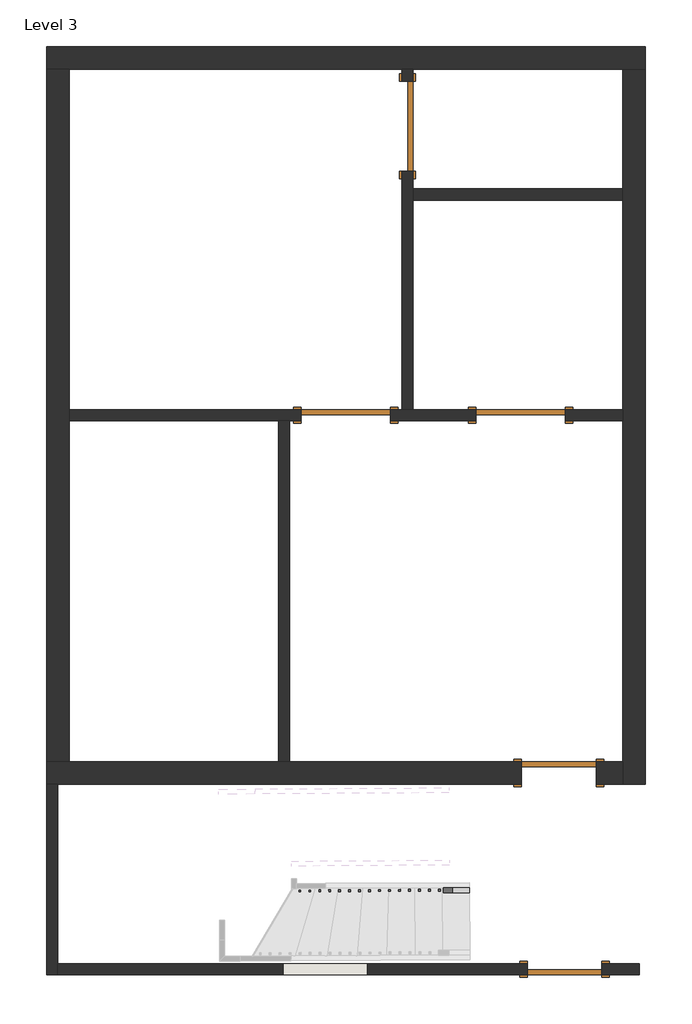
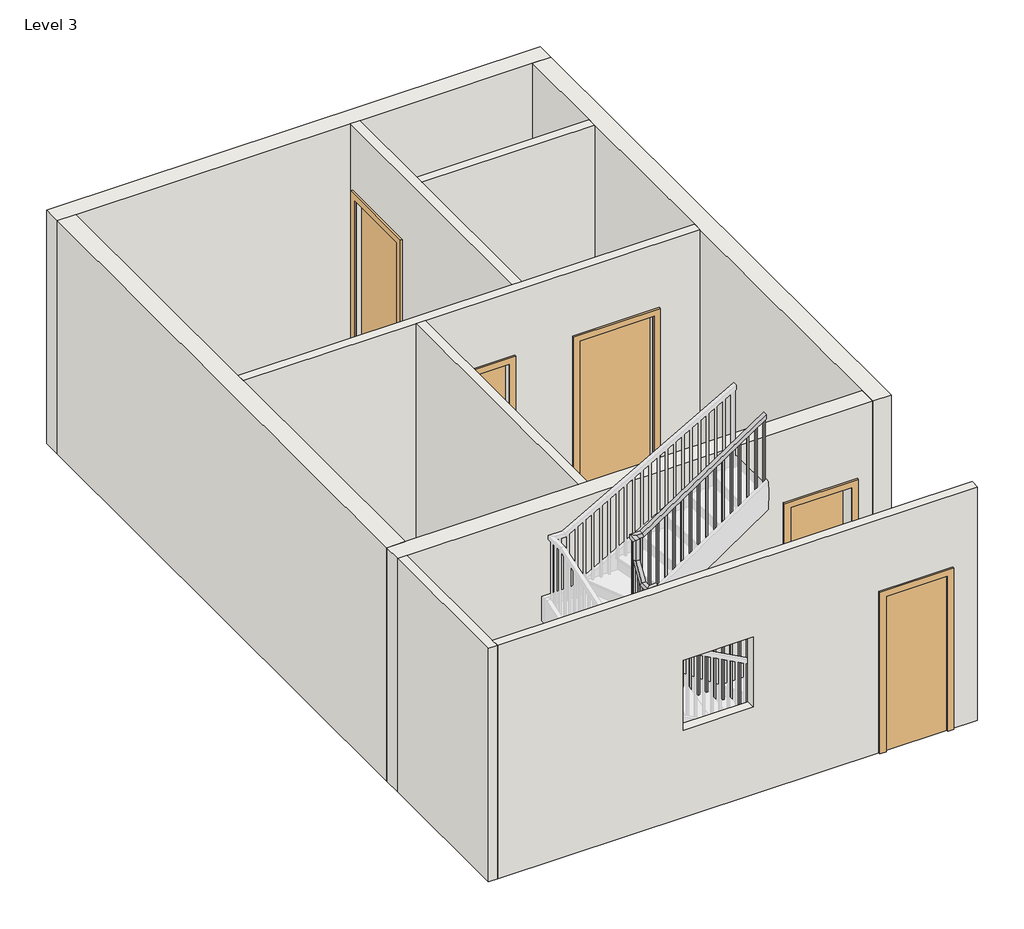
# One storey, part 1 of 2: 10 walls, 5 doors, 1 railing.
"""IFC4 building model written with IfcOpenShell, lengths in millimetres."""

from ifc_helpers import new_model, si_unit, frame, origin, place, context, project, spatial, polyline, outline, extrude, faceted_brep, transform, mapped, element, save
from components import door_a1484949, door_d8f5dbb5, door_e5f9f3c4, door_305aa2a5

model = new_model("IFC4")

# Units and contexts
model_context = context("Model", 3, world=origin())
ifc_project = project(units=[si_unit("LENGTHUNIT", "METRE", prefix="MILLI")], contexts=[model_context])

# Site, building, storey
site = spatial("IfcSite", under=ifc_project)
building = spatial("IfcBuilding", under=site)
storey = spatial("IfcBuildingStorey", under=building, Name="Level 3", Elevation=3200.4)

# Doors
placement = place(None, origin())
door_shape = door_a1484949(model_context)
element("IfcDoor", 1, ObjectType="Single-Flush : 30\" x 80\"", at=placement, inside=storey, context=model_context, shape_type="MappedRepresentation", body=[
    mapped(door_shape, transform((792.5410386, -2372.0109248, 3200.4), x_axis=(1.0, 0.0, 0.0), y_axis=(0.0, 1.0, 0.0), z_axis=(0.0, 0.0, 1.0))),
])
door_2_shape = door_d8f5dbb5(model_context)
element("IfcDoor", 2, ObjectType="Single-Flush : 30\" x 80\"", at=placement, inside=storey, context=model_context, shape_type="MappedRepresentation", body=[
    mapped(door_2_shape, transform((849.6910386, -4372.2609248, 3200.4), x_axis=(-1.0, 0.0, 0.0), y_axis=(0.0, -1.0, 0.0), z_axis=(0.0, 0.0, 1.0))),
])
door_3_shape = door_e5f9f3c4(model_context)
element("IfcDoor", 3, ObjectType="Single-Flush : 36\" x 84\"", at=placement, inside=storey, context=model_context, shape_type="MappedRepresentation", body=[
    mapped(door_3_shape, transform((-750.5089614, 4209.7640752, 3200.4), x_axis=(0.0, -1.0, 0.0), y_axis=(1.0, 0.0, 0.0), z_axis=(0.0, 0.0, 1.0))),
])
door_4_shape = door_305aa2a5(model_context)
element("IfcDoor", 4, ObjectType="Single-Flush : 36\" x 84\"", at=placement, inside=storey, context=model_context, shape_type="MappedRepresentation", body=[
    mapped(door_4_shape, transform((402.0160386, 1266.5390752, 3200.4), x_axis=(-1.0, 0.0, 0.0), y_axis=(0.0, -1.0, 0.0), z_axis=(0.0, 0.0, 1.0))),
])
element("IfcDoor", 5, ObjectType="Single-Flush : 36\" x 84\"", at=placement, inside=storey, context=model_context, shape_type="MappedRepresentation", body=[
    mapped(door_4_shape, transform((-1379.1589614, 1266.5390752, 3200.4), x_axis=(-1.0, 0.0, 0.0), y_axis=(0.0, -1.0, 0.0), z_axis=(0.0, 0.0, 1.0))),
])

# Railing
element("IfcRailing", 6, ObjectType="Handrail - Rectangular", at=placement, inside=storey, context=model_context, shape_type="SolidModel", body=[
    faceted_brep([(-120.3816305, -3590.4209536, 4284.1333333), (-120.3816305, -3590.4209536, 4222.9630107), (-120.6930289, -3539.621908, 4222.9630107), (-120.6930289, -3539.621908, 4284.1333333), (-1854.5612186, -3601.0514854, 5447.4182998), (-1905.3602642, -3601.3628839, 5420.3238978), (-1905.6716627, -3550.5638383, 5420.3238978), (-1854.8726171, -3550.2524399, 5447.4182998), (-1854.5612186, -3601.0514854, 5669.6829276), (-1905.3602642, -3601.3628839, 5618.8829276), (-1905.6716627, -3550.5638383, 5618.8829276), (-1854.8726171, -3550.2524399, 5669.6829276), (-1981.5588325, -3601.8299816, 5669.6829276), (-1981.5588325, -3601.8299816, 5618.8829276), (-1931.0711854, -3550.7195376, 5618.8829276), (-1931.0711854, -3550.7195376, 5669.6829276), (-1982.3373287, -3474.8323677, 5669.6829276), (-1982.5128182, -3446.2044317, 5618.8829276), (-1931.7137726, -3445.8930332, 5618.8829276), (-1931.5382832, -3474.5209692, 5669.6829276), (-1983.1158249, -3347.8347538, 5879.4434812), (-1983.4272234, -3297.0357082, 5865.2632575), (-1932.6281778, -3296.7243097, 5865.2632575), (-1932.3167793, -3347.5233553, 5879.4434812), (-1983.1158249, -3347.8347538, 6150.8951436), (-1983.4272234, -3297.0357082, 6100.0951436), (-1932.6281778, -3296.7243097, 6100.0951436), (-1932.3167793, -3347.5233553, 6150.8951436), (-1983.8943211, -3220.8371398, 6150.8951436), (-1983.8943211, -3220.8371398, 6100.0951436), (-1932.783877, -3271.3247869, 6100.0951436), (-1932.783877, -3271.3247869, 6150.8951436), (-1856.8967072, -3220.0586437, 6150.8951436), (-1841.6341703, -3219.9650842, 6100.0951436), (-1841.3227719, -3270.7641298, 6100.0951436), (-1856.5853087, -3270.8576892, 6150.8951436), (-324.9523945, -3210.6678153, 7162.8), (-324.6409961, -3261.4668609, 7162.8), (-324.6409961, -3261.4668609, 7101.9185401), (-324.9523945, -3210.6678153, 7101.9185401)], [[[0, 1, 2, 3]], [[1, 0, 4, 5]], [[2, 1, 5, 6]], [[3, 2, 6, 7]], [[0, 3, 7, 4]], [[5, 4, 8, 9]], [[6, 5, 9, 10]], [[7, 6, 10, 11]], [[4, 7, 11, 8]], [[9, 8, 12, 13]], [[10, 9, 13, 14]], [[11, 10, 14, 15]], [[8, 11, 15, 12]], [[13, 12, 16, 17]], [[14, 13, 17, 18]], [[15, 14, 18, 19]], [[12, 15, 19, 16]], [[17, 16, 20, 21]], [[18, 17, 21, 22]], [[19, 18, 22, 23]], [[16, 19, 23, 20]], [[21, 20, 24, 25]], [[22, 21, 25, 26]], [[23, 22, 26, 27]], [[20, 23, 27, 24]], [[25, 24, 28, 29]], [[26, 25, 29, 30]], [[27, 26, 30, 31]], [[24, 27, 31, 28]], [[29, 28, 32, 33]], [[30, 29, 33, 34]], [[31, 30, 34, 35]], [[28, 31, 35, 32]], [[36, 37, 38, 39]], [[33, 32, 36, 39]], [[34, 33, 39, 38]], [[35, 34, 38, 37]], [[32, 35, 37, 36]]]),
    extrude(outline(polyline([(222.3085098, -19.05), (234.8914903, 0.0), (1246.1854534, 0.0), (1246.1854534, -19.05), (222.3085098, -19.05)])), frame((-342.2360746, -3245.6994205, 7325.2521201), z_axis=(-0.00612989118043648, 0.9999812120405643, 0.0), x_axis=(0.0, 0.0, -1.0)), (0.0, 0.0, 1.0), 19.05),
    extrude(outline(polyline([(222.3085098, -19.0499999), (234.8914902, 0.0), (1179.0762243, 0.0), (1179.0762243, -19.0499999), (222.3085098, -19.0499999)])), frame((-443.8341657, -3246.3222175, 7258.142891), z_axis=(-0.00612989118043648, 0.9999812120405643, 0.0), x_axis=(0.0, 0.0, -1.0)), (0.0, 0.0, 1.0), 19.05),
    extrude(outline(polyline([(222.3085098, -19.05), (234.8914902, 0.0), (1111.9669952, 0.0), (1111.9669952, -19.05), (222.3085098, -19.05)])), frame((-545.4322569, -3246.9450144, 7191.0336619), z_axis=(-0.00612989118043648, 0.9999812120405643, 0.0), x_axis=(0.0, 0.0, -1.0)), (0.0, 0.0, 1.0), 19.05),
    extrude(outline(polyline([(222.3085098, -19.05), (234.8914902, 0.0), (1214.1910995, 0.0), (1214.1910995, -19.05), (222.3085098, -19.05)])), frame((-647.030348, -3247.5678114, 7123.9244328), z_axis=(-0.00612989118043648, 0.9999812120405643, 0.0), x_axis=(0.0, 0.0, -1.0)), (0.0, 0.0, 1.0), 19.05),
    extrude(outline(polyline([(222.3085098, -19.05), (234.8914902, 0.0), (1147.0818704, 0.0), (1147.0818704, -19.05), (222.3085098, -19.05)])), frame((-748.6284392, -3248.1906083, 7056.8152037), z_axis=(-0.00612989118043648, 0.9999812120405643, 0.0), x_axis=(0.0, 0.0, -1.0)), (0.0, 0.0, 1.0), 19.05),
    extrude(outline(polyline([(222.3085098, -19.05), (234.8914902, 0.0), (1079.9726413, 0.0), (1079.9726413, -19.05), (222.3085098, -19.05)])), frame((-850.2265303, -3248.8134053, 6989.7059746), z_axis=(-0.00612989118043648, 0.9999812120405643, 0.0), x_axis=(0.0, 0.0, -1.0)), (0.0, 0.0, 1.0), 19.05),
    extrude(outline(polyline([(222.3085098, -19.05), (234.8914902, 0.0), (1182.1967455, 0.0), (1182.1967455, -19.05), (222.3085098, -19.05)])), frame((-951.8246215, -3249.4362022, 6922.5967455), z_axis=(-0.00612989118043648, 0.9999812120405643, 0.0), x_axis=(0.0, 0.0, -1.0)), (0.0, 0.0, 1.0), 19.05),
    extrude(outline(polyline([(222.3085097, -19.05), (234.8914902, 0.0), (1115.0875164, 0.0), (1115.0875164, -19.05), (222.3085097, -19.05)])), frame((-1053.4227126, -3250.0589992, 6855.4875164), z_axis=(-0.00612989118043648, 0.9999812120405643, 0.0), x_axis=(0.0, 0.0, -1.0)), (0.0, 0.0, 1.0), 19.05),
    extrude(outline(polyline([(222.3085097, -19.0499999), (234.8914902, 0.0), (1047.9782873, 0.0), (1047.9782873, -19.0499999), (222.3085097, -19.0499999)])), frame((-1155.0208037, -3250.6817961, 6788.3782873), z_axis=(-0.00612989118043648, 0.9999812120405643, 0.0), x_axis=(0.0, 0.0, -1.0)), (0.0, 0.0, 1.0), 19.05),
    extrude(outline(polyline([(222.3085097, -19.05), (234.8914902, 0.0), (1150.2023915, 0.0), (1150.2023915, -19.05), (222.3085097, -19.05)])), frame((-1256.6188949, -3251.304593, 6721.2690582), z_axis=(-0.00612989118043648, 0.9999812120405643, 0.0), x_axis=(0.0, 0.0, -1.0)), (0.0, 0.0, 1.0), 19.05),
    extrude(outline(polyline([(222.3085098, -19.05), (234.8914903, 0.0), (1083.0931625, 0.0), (1083.0931625, -19.05), (222.3085098, -19.05)])), frame((-1358.216986, -3251.92739, 6654.1598292), z_axis=(-0.00612989118043648, 0.9999812120405643, 0.0), x_axis=(0.0, 0.0, -1.0)), (0.0, 0.0, 1.0), 19.05),
    extrude(outline(polyline([(222.3085098, -19.05), (234.8914903, 0.0), (1185.3172668, 0.0), (1185.3172668, -19.05), (222.3085098, -19.05)])), frame((-1459.8150772, -3252.5501869, 6587.0506001), z_axis=(-0.00612989118043648, 0.9999812120405643, 0.0), x_axis=(0.0, 0.0, -1.0)), (0.0, 0.0, 1.0), 19.05),
    extrude(outline(polyline([(222.3085098, -19.05), (234.8914903, 0.0), (1118.2080377, 0.0), (1118.2080377, -19.05), (222.3085098, -19.05)])), frame((-1561.4131683, -3253.1729839, 6519.941371), z_axis=(-0.00612989118043648, 0.9999812120405643, 0.0), x_axis=(0.0, 0.0, -1.0)), (0.0, 0.0, 1.0), 19.05),
    extrude(outline(polyline([(222.3085098, -19.05), (234.8914902, 0.0), (1051.0988086, 0.0), (1051.0988086, -19.05), (222.3085098, -19.05)])), frame((-1663.0112595, -3253.7957808, 6452.8321419), z_axis=(-0.00612989118043648, 0.9999812120405643, 0.0), x_axis=(0.0, 0.0, -1.0)), (0.0, 0.0, 1.0), 19.05),
    extrude(outline(polyline([(222.3085098, -19.05), (234.8914902, 0.0), (1153.3229128, 0.0), (1153.3229128, -19.05), (222.3085098, -19.05)])), frame((-1764.6093506, -3254.4185778, 6385.7229128), z_axis=(-0.00612989118043648, 0.9999812120405643, 0.0), x_axis=(0.0, 0.0, -1.0)), (0.0, 0.0, 1.0), 19.05),
    extrude(outline(polyline([(222.3085098, -19.05), (234.8914902, 0.0), (1086.2136837, 0.0), (1086.2136837, -19.05), (222.3085098, -19.05)])), frame((-1866.2074418, -3255.0413747, 6318.6136837), z_axis=(-0.00612989118043648, 0.9999812120405643, 0.0), x_axis=(0.0, 0.0, -1.0)), (0.0, 0.0, 1.0), 19.05),
    extrude(outline(polyline([(-1948.6001916, -3280.94692), (-1967.6498337, -3281.0636944), (-1967.7666081, -3262.0140523), (-1948.716966, -3261.8972779), (-1948.6001916, -3280.94692)])), frame((0.0, 0.0, 5063.0666667), z_axis=(0.0, 0.0, 1.0), x_axis=(1.0, 0.0, 0.0)), (0.0, 0.0, 1.0), 1037.0284769),
    extrude(outline(polyline([(244.3320415, -19.05), (212.8679585, 0.0), (1074.2735921, 0.0), (1074.2735921, -19.05), (244.3320415, -19.05)])), frame((-1967.1438111, -3363.6121435, 5968.0069254), z_axis=(0.9999812120405644, 0.006129891180436036, 0.0), x_axis=(0.0, 0.0, -1.0)), (0.0, 0.0, 1.0), 19.05),
    extrude(outline(polyline([(244.3320415, -19.05), (212.8679585, 0.0), (1075.7984825, 0.0), (1075.7984825, -19.05), (244.3320415, -19.05)])), frame((-1966.5210142, -3465.2102346, 5800.1984825), z_axis=(0.9999812120405644, 0.006129891180436036, 0.0), x_axis=(0.0, 0.0, -1.0)), (0.0, 0.0, 1.0), 19.05),
    extrude(outline(polyline([(-1939.8365364, -3566.6485675), (-1939.719762, -3585.6982096), (-1958.7694041, -3585.814984), (-1958.8861785, -3566.7653419), (-1939.8365364, -3566.6485675)])), frame((0.0, 0.0, 4555.0666667), z_axis=(0.0, 0.0, 1.0), x_axis=(1.0, 0.0, 0.0)), (0.0, 0.0, 1.0), 1063.816261),
    extrude(outline(polyline([(234.9892351, -19.05), (222.2107648, 0.0), (1224.4109792, 0.0), (1224.4109792, -19.05), (234.9892351, -19.05)])), frame((-1857.171313, -3585.1921871, 5610.1443125), z_axis=(-0.006129891180436334, 0.9999812120405643, 0.0), x_axis=(0.0, 0.0, -1.0)), (0.0, 0.0, 1.0), 19.05),
    extrude(outline(polyline([(234.9892352, -19.05), (222.2107649, 0.0), (1156.259138, 0.0), (1156.259138, -19.05), (234.9892352, -19.05)])), frame((-1755.5732218, -3584.5693901, 5541.9924713), z_axis=(-0.006129891180436334, 0.9999812120405643, 0.0), x_axis=(0.0, 0.0, -1.0)), (0.0, 0.0, 1.0), 19.05),
    extrude(outline(polyline([(234.9892351, -19.05), (222.2107649, 0.0), (1257.44063, 0.0), (1257.44063, -19.05), (234.9892351, -19.05)])), frame((-1653.9751307, -3583.9465932, 5473.84063), z_axis=(-0.006129891180436334, 0.9999812120405643, 0.0), x_axis=(0.0, 0.0, -1.0)), (0.0, 0.0, 1.0), 19.05),
    extrude(outline(polyline([(234.9892351, -19.05), (222.2107649, 0.0), (1189.2887887, 0.0), (1189.2887887, -19.05), (234.9892351, -19.05)])), frame((-1552.3770395, -3583.3237962, 5405.6887887), z_axis=(-0.006129891180436334, 0.9999812120405643, 0.0), x_axis=(0.0, 0.0, -1.0)), (0.0, 0.0, 1.0), 19.05),
    extrude(outline(polyline([(234.9892351, -19.05), (222.2107649, 0.0), (1290.4702807, 0.0), (1290.4702807, -19.05), (234.9892351, -19.05)])), frame((-1450.7789484, -3582.7009993, 5337.5369474), z_axis=(-0.006129891180436334, 0.9999812120405643, 0.0), x_axis=(0.0, 0.0, -1.0)), (0.0, 0.0, 1.0), 19.05),
    extrude(outline(polyline([(234.9892351, -19.0499999), (222.2107649, 0.0), (1222.3184394, 0.0), (1222.3184394, -19.0499999), (234.9892351, -19.0499999)])), frame((-1349.1808572, -3582.0782024, 5269.3851061), z_axis=(-0.006129891180436334, 0.9999812120405643, 0.0), x_axis=(0.0, 0.0, -1.0)), (0.0, 0.0, 1.0), 19.05),
    extrude(outline(polyline([(234.9892351, -19.05), (222.2107648, 0.0), (1154.1665981, 0.0), (1154.1665981, -19.05), (234.9892351, -19.05)])), frame((-1247.5827661, -3581.4554054, 5201.2332648), z_axis=(-0.006129891180436334, 0.9999812120405643, 0.0), x_axis=(0.0, 0.0, -1.0)), (0.0, 0.0, 1.0), 19.05),
    extrude(outline(polyline([(234.9892352, -19.05), (222.2107649, 0.0), (1255.3480903, 0.0), (1255.3480903, -19.05), (234.9892352, -19.05)])), frame((-1145.984675, -3580.8326085, 5133.0814236), z_axis=(-0.006129891180436334, 0.9999812120405643, 0.0), x_axis=(0.0, 0.0, -1.0)), (0.0, 0.0, 1.0), 19.05),
    extrude(outline(polyline([(234.9892351, -19.05), (222.2107649, 0.0), (1187.196249, 0.0), (1187.196249, -19.05), (234.9892351, -19.05)])), frame((-1044.3865838, -3580.2098115, 5064.9295823), z_axis=(-0.006129891180436334, 0.9999812120405643, 0.0), x_axis=(0.0, 0.0, -1.0)), (0.0, 0.0, 1.0), 19.05),
    extrude(outline(polyline([(234.9892351, -19.05), (222.2107649, 0.0), (1288.377741, 0.0), (1288.377741, -19.05), (234.9892351, -19.05)])), frame((-942.7884927, -3579.5870146, 4996.777741), z_axis=(-0.006129891180436334, 0.9999812120405643, 0.0), x_axis=(0.0, 0.0, -1.0)), (0.0, 0.0, 1.0), 19.05),
    extrude(outline(polyline([(234.9892351, -19.05), (222.2107649, 0.0), (1220.2258997, 0.0), (1220.2258997, -19.05), (234.9892351, -19.05)])), frame((-841.1904015, -3578.9642176, 4928.6258997), z_axis=(-0.006129891180436334, 0.9999812120405643, 0.0), x_axis=(0.0, 0.0, -1.0)), (0.0, 0.0, 1.0), 19.05),
    extrude(outline(polyline([(234.9892351, -19.05), (222.2107649, 0.0), (1152.0740584, 0.0), (1152.0740584, -19.05), (234.9892351, -19.05)])), frame((-739.5923104, -3578.3414207, 4860.4740584), z_axis=(-0.006129891180436334, 0.9999812120405643, 0.0), x_axis=(0.0, 0.0, -1.0)), (0.0, 0.0, 1.0), 19.05),
    extrude(outline(polyline([(234.9892351, -19.0499999), (222.2107648, 0.0), (1253.2555504, 0.0), (1253.2555504, -19.0499999), (234.9892351, -19.0499999)])), frame((-637.9942192, -3577.7186237, 4792.3222171), z_axis=(-0.006129891180436334, 0.9999812120405643, 0.0), x_axis=(0.0, 0.0, -1.0)), (0.0, 0.0, 1.0), 19.05),
    extrude(outline(polyline([(234.9892352, -19.05), (222.2107649, 0.0), (1185.1037092, 0.0), (1185.1037092, -19.05), (234.9892352, -19.05)])), frame((-536.3961281, -3577.0958268, 4724.1703759), z_axis=(-0.006129891180436334, 0.9999812120405643, 0.0), x_axis=(0.0, 0.0, -1.0)), (0.0, 0.0, 1.0), 19.05),
    extrude(outline(polyline([(234.9892351, -19.05), (222.2107649, 0.0), (1116.9518679, 0.0), (1116.9518679, -19.05), (234.9892351, -19.05)])), frame((-434.798037, -3576.4730299, 4656.0185346), z_axis=(-0.006129891180436334, 0.9999812120405643, 0.0), x_axis=(0.0, 0.0, -1.0)), (0.0, 0.0, 1.0), 19.05),
    extrude(outline(polyline([(234.9892351, -19.05), (222.2107649, 0.0), (1218.13336, 0.0), (1218.13336, -19.05), (234.9892351, -19.05)])), frame((-333.1999458, -3575.8502329, 4587.8666933), z_axis=(-0.006129891180436334, 0.9999812120405643, 0.0), x_axis=(0.0, 0.0, -1.0)), (0.0, 0.0, 1.0), 19.05),
    extrude(outline(polyline([(234.9892351, -19.05), (222.2107649, 0.0), (1149.9815187, 0.0), (1149.9815187, -19.05), (234.9892351, -19.05)])), frame((-231.6018547, -3575.227436, 4519.714852), z_axis=(-0.006129891180436334, 0.9999812120405643, 0.0), x_axis=(0.0, 0.0, -1.0)), (0.0, 0.0, 1.0), 19.05),
    extrude(outline(polyline([(-1948.7558908, -3255.5473972), (-1967.8055329, -3255.6641716), (-1967.9223073, -3236.6145296), (-1948.8726652, -3236.4977551), (-1948.7558908, -3255.5473972)])), frame((0.0, 0.0, 5063.0666667), z_axis=(0.0, 0.0, 1.0), x_axis=(1.0, 0.0, 0.0)), (0.0, 0.0, 1.0), 1037.0284769),
    extrude(outline(polyline([(-1946.8485752, -3566.6915513), (-1946.7318007, -3585.7411934), (-1965.7814428, -3585.8579679), (-1965.8982173, -3566.8083258), (-1946.8485752, -3566.6915513)])), frame((0.0, 0.0, 4555.0666667), z_axis=(0.0, 0.0, 1.0), x_axis=(1.0, 0.0, 0.0)), (0.0, 0.0, 1.0), 1063.816261),
    extrude(outline(polyline([(222.3085098, -19.05), (234.8914902, 0.0), (1245.1603832, 0.0), (1245.1603832, -19.05), (222.3085098, -19.05)])), frame((-343.7879502, -3245.7089335, 7324.2270499), z_axis=(-0.00612989118043648, 0.9999812120405643, 0.0), x_axis=(0.0, 0.0, -1.0)), (0.0, 0.0, 1.0), 19.05),
    extrude(outline(polyline([(234.9892351, -19.05), (222.2107648, 0.0), (1088.2189125, 0.0), (1088.2189125, -19.05), (234.9892351, -19.05)])), frame((-139.5285846, -3574.6630262, 4457.9522458), z_axis=(-0.006129891180436334, 0.9999812120405643, 0.0), x_axis=(0.0, 0.0, -1.0)), (0.0, 0.0, 1.0), 19.05),
])

# Walls
element("IfcWall", 7, ObjectType="4.5\"", at=placement, inside=storey, context=model_context, shape_type="Brep", body=[
    faceted_brep([(-807.6589614, 3752.5640752, 5334.0), (-807.6589614, 3752.5640752, 3200.4), (-807.6589614, 1323.6890752, 3200.4), (-807.6589614, 1323.6890752, 6248.4), (-807.6589614, 4790.7890752, 6248.4), (-807.6589614, 4790.7890752, 3200.4), (-807.6589614, 4666.9640752, 3200.4), (-807.6589614, 4666.9640752, 5334.0), (-693.3589614, 1323.6890752, 3200.4), (-693.3589614, 3457.2890752, 3200.4), (-693.3589614, 3571.5890752, 3200.4), (-693.3589614, 3752.5640752, 3200.4), (-693.3589614, 3752.5640752, 5334.0), (-693.3589614, 4666.9640752, 5334.0), (-693.3589614, 4666.9640752, 3200.4), (-693.3589614, 4790.7890752, 3200.4), (-693.3589614, 4790.7890752, 6248.4), (-693.3589614, 3571.5890752, 6248.4), (-693.3589614, 3457.2890752, 6248.4), (-693.3589614, 1323.6890752, 6248.4)], [[[0, 1, 2, 3, 4, 5, 6, 7]], [[8, 9, 10, 11, 12, 13, 14, 15, 16, 17, 18, 19]], [[6, 5, 15, 14]], [[2, 1, 11, 10, 9, 8]], [[5, 4, 16, 15]], [[3, 2, 8, 19]], [[12, 11, 1, 0]], [[13, 12, 0, 7]], [[14, 13, 7, 6]], [[4, 3, 19, 18, 17, 16]]]),
])
element("IfcWall", 8, ObjectType="4.5\"", at=placement, inside=storey, context=model_context, shape_type="SweptSolid", body=[
    extrude(outline(polyline([(-693.3589614, 3571.5890752), (1440.2410386, 3571.5890752), (1440.2410386, 3457.2890752), (-693.3589614, 3457.2890752), (-693.3589614, 3571.5890752)])), frame((0.0, 0.0, 3200.4), z_axis=(0.0, 0.0, 1.0), x_axis=(1.0, 0.0, 0.0)), (0.0, 0.0, 1.0), 3048.0),
])
element("IfcWall", 9, ObjectType="4.5\"", at=placement, inside=storey, context=model_context, shape_type="Brep", body=[
    faceted_brep([(-4198.5589614, 1209.3890752, 3200.4), (-2064.9589614, 1209.3890752, 3200.4), (-1950.6589614, 1209.3890752, 3200.4), (-1836.3589614, 1209.3890752, 3200.4), (-1836.3589614, 1209.3890752, 5334.0), (-921.9589614, 1209.3890752, 5334.0), (-921.9589614, 1209.3890752, 3200.4), (-55.1839614, 1209.3890752, 3200.4), (-55.1839614, 1209.3890752, 5334.0), (859.2160386, 1209.3890752, 5334.0), (859.2160386, 1209.3890752, 3200.4), (1440.2410386, 1209.3890752, 3200.4), (1440.2410386, 1209.3890752, 6248.4), (-1950.6589614, 1209.3890752, 6248.4), (-2064.9589614, 1209.3890752, 6248.4), (-4198.5589614, 1209.3890752, 6248.4), (-1836.3589614, 1323.6890752, 5334.0), (-1836.3589614, 1323.6890752, 3200.4), (-4198.5589614, 1323.6890752, 3200.4), (-4198.5589614, 1323.6890752, 6248.4), (-807.6589614, 1323.6890752, 6248.4), (-693.3589614, 1323.6890752, 6248.4), (1440.2410386, 1323.6890752, 6248.4), (1440.2410386, 1323.6890752, 3200.4), (859.2160386, 1323.6890752, 3200.4), (859.2160386, 1323.6890752, 5334.0), (-55.1839614, 1323.6890752, 5334.0), (-55.1839614, 1323.6890752, 3200.4), (-693.3589614, 1323.6890752, 3200.4), (-807.6589614, 1323.6890752, 3200.4), (-921.9589614, 1323.6890752, 3200.4), (-921.9589614, 1323.6890752, 5334.0)], [[[0, 1, 2, 3, 4, 5, 6, 7, 8, 9, 10, 11, 12, 13, 14, 15]], [[16, 17, 18, 19, 20, 21, 22, 23, 24, 25, 26, 27, 28, 29, 30, 31]], [[24, 23, 11, 10]], [[18, 17, 3, 2, 1, 0]], [[30, 29, 28, 27, 7, 6]], [[12, 11, 23, 22]], [[0, 15, 19, 18]], [[8, 7, 27, 26]], [[9, 8, 26, 25]], [[10, 9, 25, 24]], [[4, 3, 17, 16]], [[5, 4, 16, 31]], [[6, 5, 31, 30]], [[15, 14, 13, 12, 22, 21, 20, 19]]]),
])
element("IfcWall", 10, ObjectType="4.5\"", at=placement, inside=storey, context=model_context, shape_type="SweptSolid", body=[
    extrude(outline(polyline([(-2064.9589614, -2257.7109248), (-2064.9589614, 1209.3890752), (-1950.6589614, 1209.3890752), (-1950.6589614, -2257.7109248), (-2064.9589614, -2257.7109248)])), frame((0.0, 0.0, 3200.4), z_axis=(0.0, 0.0, 1.0), x_axis=(1.0, 0.0, 0.0)), (0.0, 0.0, 1.0), 3048.0),
])
element("IfcWall", 11, ObjectType="4.5\"", at=placement, inside=storey, context=model_context, shape_type="Brep", body=[
    faceted_brep([(-4427.1589614, -2486.3109248, 3200.4), (-4427.1589614, -4429.4109248, 3200.4), (-4427.1589614, -4429.4109248, 6248.4), (-4427.1589614, -2486.3109248, 6248.4), (-4312.8589614, -2486.3109248, 3200.4), (-4312.8589614, -2486.3109248, 6248.4), (-4312.8589614, -4315.1109248, 6248.4), (-4312.8589614, -4429.4109248, 6248.4), (-4312.8589614, -4429.4109248, 3200.4), (-4312.8589614, -4315.1109248, 3200.4)], [[[0, 1, 2, 3]], [[4, 5, 6, 7, 8, 9]], [[1, 0, 4, 9, 8]], [[3, 2, 7, 6, 5]], [[0, 3, 5, 4]], [[2, 1, 8, 7]]]),
])
element("IfcWall", 12, ObjectType="4.5\"", at=placement, inside=storey, context=model_context, shape_type="SweptSolid", body=[
    extrude(outline(polyline([(3200.4, -4312.8589614), (3200.4, 468.6910386), (5232.4, 468.6910386), (5232.4, 1230.6910386), (3200.4, 1230.6910386), (3200.4, 1611.6910386), (6248.4, 1611.6910386), (6248.4, -4312.8589614), (3200.4, -4312.8589614)]), holes=[polyline([(5254.5695631, -2020.5089614), (5254.5695631, -1156.9089614), (4340.1695631, -1156.9089614), (4340.1695631, -2020.5089614), (5254.5695631, -2020.5089614)])]), frame((0.0, -4429.4109248, 0.0), z_axis=(0.0, 1.0, 0.0), x_axis=(0.0, 0.0, 1.0)), (0.0, 0.0, 1.0), 114.3),
])
element("IfcWall", 13, ObjectType="9\"", at=placement, inside=storey, context=model_context, shape_type="Brep", body=[
    faceted_brep([(-4427.1589614, 4790.7890752, 3200.4), (-4198.5589614, 4790.7890752, 3200.4), (-807.6589614, 4790.7890752, 3200.4), (-693.3589614, 4790.7890752, 3200.4), (1440.2410386, 4790.7890752, 3200.4), (1668.8410386, 4790.7890752, 3200.4), (1668.8410386, 4790.7890752, 6248.4), (1440.2410386, 4790.7890752, 6248.4), (-693.3589614, 4790.7890752, 6248.4), (-807.6589614, 4790.7890752, 6248.4), (-4198.5589614, 4790.7890752, 6248.4), (-4427.1589614, 4790.7890752, 6248.4), (-4427.1589614, 5019.3890752, 3200.4), (-4427.1589614, 5019.3890752, 6248.4), (1668.8410386, 5019.3890752, 6248.4), (1668.8410386, 5019.3890752, 3200.4)], [[[0, 1, 2, 3, 4, 5, 6, 7, 8, 9, 10, 11]], [[12, 13, 14, 15]], [[5, 4, 3, 2, 1, 0, 12, 15]], [[6, 5, 15, 14]], [[0, 11, 13, 12]], [[11, 10, 9, 8, 7, 6, 14, 13]]]),
])
element("IfcWall", 14, ObjectType="9\"", at=placement, inside=storey, context=model_context, shape_type="Brep", body=[
    faceted_brep([(1440.2410386, 4790.7890752, 3200.4), (1440.2410386, 3571.5890752, 3200.4), (1440.2410386, 3457.2890752, 3200.4), (1440.2410386, 1323.6890752, 3200.4), (1440.2410386, 1209.3890752, 3200.4), (1440.2410386, -2257.7109248, 3200.4), (1440.2410386, -2486.3109248, 3200.4), (1440.2410386, -2486.3109248, 6248.4), (1440.2410386, -2257.7109248, 6248.4), (1440.2410386, 1209.3890752, 6248.4), (1440.2410386, 1323.6890752, 6248.4), (1440.2410386, 3457.2890752, 6248.4), (1440.2410386, 3571.5890752, 6248.4), (1440.2410386, 4790.7890752, 6248.4), (1668.8410386, 4790.7890752, 3200.4), (1668.8410386, 4790.7890752, 6248.4), (1668.8410386, -2486.3109248, 6248.4), (1668.8410386, -2486.3109248, 3200.4)], [[[0, 1, 2, 3, 4, 5, 6, 7, 8, 9, 10, 11, 12, 13]], [[14, 15, 16, 17]], [[6, 5, 4, 3, 2, 1, 0, 14, 17]], [[0, 13, 15, 14]], [[7, 6, 17, 16]], [[13, 12, 11, 10, 9, 8, 7, 16, 15]]]),
])
element("IfcWall", 15, ObjectType="9\"", at=placement, inside=storey, context=model_context, shape_type="Brep", body=[
    faceted_brep([(1440.2410386, -2257.7109248, 3200.4), (1173.5410386, -2257.7109248, 3200.4), (1173.5410386, -2257.7109248, 5232.4), (411.5410386, -2257.7109248, 5232.4), (411.5410386, -2257.7109248, 3200.4), (-1950.6589614, -2257.7109248, 3200.4), (-2064.9589614, -2257.7109248, 3200.4), (-4198.5589614, -2257.7109248, 3200.4), (-4427.1589614, -2257.7109248, 3200.4), (-4427.1589614, -2257.7109248, 6248.4), (-4198.5589614, -2257.7109248, 6248.4), (-2064.9589614, -2257.7109248, 6248.4), (-1950.6589614, -2257.7109248, 6248.4), (1440.2410386, -2257.7109248, 6248.4), (1173.5410386, -2486.3109248, 5232.4), (1173.5410386, -2486.3109248, 3200.4), (1440.2410386, -2486.3109248, 3200.4), (1440.2410386, -2486.3109248, 6248.4), (-4312.8589614, -2486.3109248, 6248.4), (-4427.1589614, -2486.3109248, 6248.4), (-4427.1589614, -2486.3109248, 3200.4), (-4312.8589614, -2486.3109248, 3200.4), (411.5410386, -2486.3109248, 3200.4), (411.5410386, -2486.3109248, 5232.4)], [[[0, 1, 2, 3, 4, 5, 6, 7, 8, 9, 10, 11, 12, 13]], [[14, 15, 16, 17, 18, 19, 20, 21, 22, 23]], [[16, 15, 1, 0]], [[22, 21, 20, 8, 7, 6, 5, 4]], [[0, 13, 17, 16]], [[9, 8, 20, 19]], [[2, 1, 15, 14]], [[3, 2, 14, 23]], [[4, 3, 23, 22]], [[13, 12, 11, 10, 9, 19, 18, 17]]]),
])
element("IfcWall", 16, ObjectType="9\"", at=placement, inside=storey, context=model_context, shape_type="Brep", body=[
    faceted_brep([(-4198.5589614, -2257.7109248, 3200.4), (-4198.5589614, 1209.3890752, 3200.4), (-4198.5589614, 1323.6890752, 3200.4), (-4198.5589614, 4790.7890752, 3200.4), (-4198.5589614, 4790.7890752, 6248.4), (-4198.5589614, 1323.6890752, 6248.4), (-4198.5589614, 1209.3890752, 6248.4), (-4198.5589614, -2257.7109248, 6248.4), (-4427.1589614, -2257.7109248, 3200.4), (-4427.1589614, -2257.7109248, 6248.4), (-4427.1589614, 4790.7890752, 6248.4), (-4427.1589614, 4790.7890752, 3200.4)], [[[0, 1, 2, 3, 4, 5, 6, 7]], [[8, 9, 10, 11]], [[3, 2, 1, 0, 8, 11]], [[0, 7, 9, 8]], [[4, 3, 11, 10]], [[7, 6, 5, 4, 10, 9]]]),
])

save(model, "model.ifc")

# Revit data of these elements
# Type "Single-Flush : 30\" x 80\""
#   Type Mark = "5"
#   Construction Type Id = "MDOOR"
#   Assembly Code = "C1020"
#   Analytic Construction = "Metal"
#   Thickness = 0' - 2"
#   Heat Transfer Coefficient (U) = 0.651978 BTU/(h·ft²·°F)
#   Height = 6' - 8"
#   Trim Projection Ext = 0' - 1"
#   Trim Projection Int = 0' - 1"
#   Trim Width = 0' - 3"
#   Width = 2' - 6"
#   Define Thermal Properties by = 1
#   Define Thermal Properties by = 1
#   Door Material = Door - Panel
#   Frame Material = Door - Frame
#   Visual Light Transmittance = 0
#   Solar Heat Gain Coefficient = 0
#   Function = (empty or 0)
#   Wall Closure = (empty or 0)
# Type "Single-Flush : 36\" x 84\""
#   Type Mark = "1"
#   Construction Type Id = "MDOOR"
#   Assembly Code = "C1020"
#   Analytic Construction = "Metal"
#   Thickness = 0' - 2"
#   Heat Transfer Coefficient (U) = 0.651978 BTU/(h·ft²·°F)
#   Height = 7' - 0"
#   Trim Projection Ext = 0' - 1"
#   Trim Projection Int = 0' - 1"
#   Trim Width = 0' - 3"
#   Width = 3' - 0"
#   Define Thermal Properties by = 1
#   Define Thermal Properties by = 1
#   Door Material = Door - Panel
#   Frame Material = Door - Frame
#   Visual Light Transmittance = 0
#   Solar Heat Gain Coefficient = 0
#   Function = (empty or 0)
#   Wall Closure = (empty or 0)
# Type "Handrail - Rectangular"
#   Assembly Code = "C2010400"
#   built-in parameter 1008612 = 0.0416667 (stored number, unit not read)
#   built-in parameter 1008611 = 0.0416667 (stored number, unit not read)
#   built-in parameter 1008609 = 0.333333 (stored number, unit not read)
#   built-in parameter 1008604 = 0.166667 (stored number, unit not read)
#   built-in parameter 1008603 = 0.166667 (stored number, unit not read)
#   Railing Height = 3' - 0"
#   built-in parameter 1008630 = 2
#   built-in parameter 1008610 = 2
#   built-in parameter 1008618 = Baluster - Square : 3/4"
# Type "4.5\""
#   Assembly Code = "B2010"
#   Layers, outside or top first: 0' - 4 1/2" no material (function 1)
# Type "9\""
#   Assembly Code = "B2010"
#   Layers, outside or top first: 0' - 9" no material (function 1)
# Elements 1, 2 (IfcDoor, "Single-Flush : 30\" x 80\"")
#   Phase Created = New Construction
#   Materials on its faces: "Door - Frame", "Door - Panel"
# Elements 3, 4, 5 (IfcDoor, "Single-Flush : 36\" x 84\"")
#   Phase Created = New Construction
#   Materials on its faces: "Door - Frame", "Door - Panel"
# Element 6 (IfcRailing, "Handrail - Rectangular")
#   Phase Created = New Construction
# Elements 7, 8, 9, 10 (IfcWall, "4.5\"")
#   Top Offset = 0' - 0"
#   Base Offset = 0' - 0"
#   Unconnected Height = 10' - 0"
#   wall height = 10' - 0"
#   Phase Created = New Construction
#   Base Constraint = Level 3
#   Materials on its faces: "Default Wall"
# Elements 11, 12 (IfcWall, "4.5\"")
#   Top Offset = 0' - 0"
#   Base Offset = 0' - 0"
#   Unconnected Height = 10' - 0"
#   wall height = 10' - 0"
#   Phase Created = New Construction
#   Base Constraint = Level 3
#   Materials on its faces: "Default Wall", "Door - Frame"
# Elements 13, 14, 15, 16 (IfcWall, "9\"")
#   Top Offset = 0' - 0"
#   Base Offset = 0' - 0"
#   Unconnected Height = 10' - 0"
#   wall height = 10' - 0"
#   Phase Created = New Construction
#   Base Constraint = Level 3
#   Materials on its faces: "Default Wall", "Door - Frame"
# Materials
#   "Door - Panel": class "Wood", colour RGB 210 159 95, transparency 0, Cost = 0
#   "Door - Frame": colour RGB 118 70 51, transparency 0, Cost = 0
#   "Default Wall": colour RGB 128 128 128, transparency 0, Cost = 0
